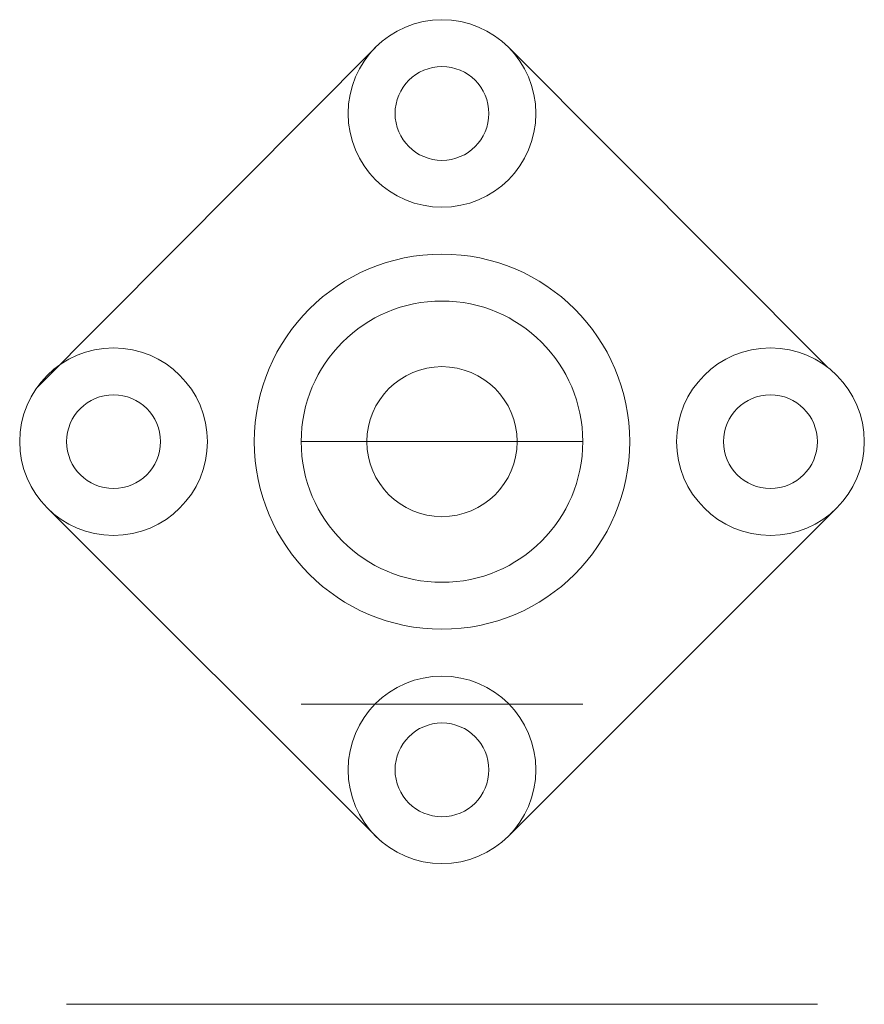
# Model space of a CAD drawing. Units: millimetres. Extents: x 105 to 195, y 120 to 225.
import ezdxf

# ---------------------------------------------------------------- set-up
doc = ezdxf.new("R2010")
doc.units = ezdxf.units.MM
doc.layers.add('M-CONS', color=8, linetype='Continuous', lineweight=13)

msp = doc.modelspace()

# ---------------------------------------------------------------- linework, layer by layer
at = {"layer": 'M-CONS'}
for p, q in [((107.12, 185.63), (143.26, 222)), ((191.39, 187.92), (157.44, 222.01)), ((143.79, 137.4), (108.28, 172.88)), ((157.43, 137.89), (192.42, 172.88))]:
    msp.add_line(p, q, dxfattribs=at)
at = {"layer": 'M-CONS', "extrusion": (0, 1, 0)}
msp.add_line((150.35, 179.95, 45), (150.35, 179.95, 53.21), dxfattribs=at)
at = {"layer": 'M-CONS'}
for centre, radius in [((150.35, 214.95), 10), ((150.35, 214.95), 5), ((150.35, 179.95), 20), ((150.35, 179.95), 20), ((150.35, 179.95), 15), ((115.35, 179.95), 10), ((185.35, 179.95), 10), ((150.35, 179.95), 8), ((115.35, 179.95), 5), ((185.35, 179.95), 5), ((150.35, 144.95), 10), ((150.35, 144.95), 5)]:
    msp.add_circle(centre, radius, dxfattribs=at)
at = {"layer": 'M-CONS', "extrusion": (0, 1, 0)}
for centre, radius in [((-150.35, 70, 179.95), 15), ((-150.35, 45, 179.95), 14.5), ((-150.35, 70, 179.95), 7.5), ((-150.35, 45, 179.95), 7.5), ((-150.35, 45, 179.95), 7.5), ((-150.35, 70, 119.95), 15), ((-150.35, 70, 119.95), 7.5)]:
    msp.add_circle(centre, radius, dxfattribs=at)
at = {"layer": 'M-CONS', "extrusion": (0, -1, 0)}
for centre, radius in [((150.35, 70, -151.95), 15), ((150.35, 70, -119.95), 40), ((120.35, 70, -119.95), 5), ((150.35, 100, -119.95), 5), ((150.35, 40, -119.95), 5), ((180.35, 70, -119.95), 5)]:
    msp.add_circle(centre, radius, dxfattribs=at)

doc.saveas('drawing.dxf')
